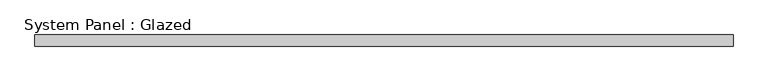
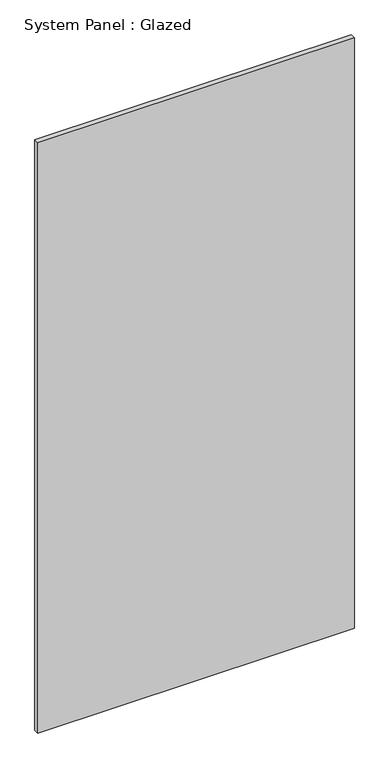
"""IFC4 building model written with IfcOpenShell, lengths in millimetres: plate geometry, System Panel : Glazed."""

from ifc_helpers import new_model, si_unit, origin, origin_with_axes, place, context, project, spatial, polyline, outline, extrude, source, transform, mapped, element, save


def system_panel_glazed_da641326(model_context):
    return source(origin(), model_context, "Body", "SweptSolid", [
        extrude(outline(polyline([(760.8925532, 24.5), (-760.8925532, 24.5), (-760.8925532, 49.5), (760.8925532, 49.5), (760.8925532, 24.5)])), origin_with_axes(), (0.0, 0.0, 1.0), 3000.0),
    ])


if __name__ == "__main__":
    model = new_model("IFC4")
    model_context = context("Model", 3, world=origin())
    ifc_project = project(units=[si_unit("LENGTHUNIT", "METRE", prefix="MILLI")], contexts=[model_context])
    site = spatial("IfcSite", under=ifc_project)
    building = spatial("IfcBuilding", under=site)
    placement = place(None, origin())
    system_panel_glazed_shape = system_panel_glazed_da641326(model_context)
    element("IfcPlate", 1, ObjectType="System Panel : Glazed", at=placement, inside=building, context=model_context, shape_type="MappedRepresentation", body=[
        mapped(system_panel_glazed_shape, transform((0.0, 0.0, 0.0), x_axis=(1.0, 0.0, 0.0), y_axis=(0.0, 1.0, 0.0), z_axis=(0.0, 0.0, 1.0))),
    ])
    save(model, "model.ifc")

# Revit data of these elements
# Type "System Panel : Glazed"
#   Keynote = "H11"
#   Construction Type Id = "GSP4R"
#   Analytic Construction = "1/8 in Pilkington single glazing"
#   Visual Light Transmittance = 0.9
#   Solar Heat Gain Coefficient = 0.86
#   Heat Transfer Coefficient (U) = 6.7069 W/(m²·K)
#   Define Thermal Properties by = 1
# Element 1 (IfcPlate, "System Panel : Glazed")
#   Materials on its faces: "Glass"
# Materials
#   "Glass": class "Glass", colour RGB 0 128 192, transparency 0.9, Description = "Soda Lime Glass", Cost = 0
